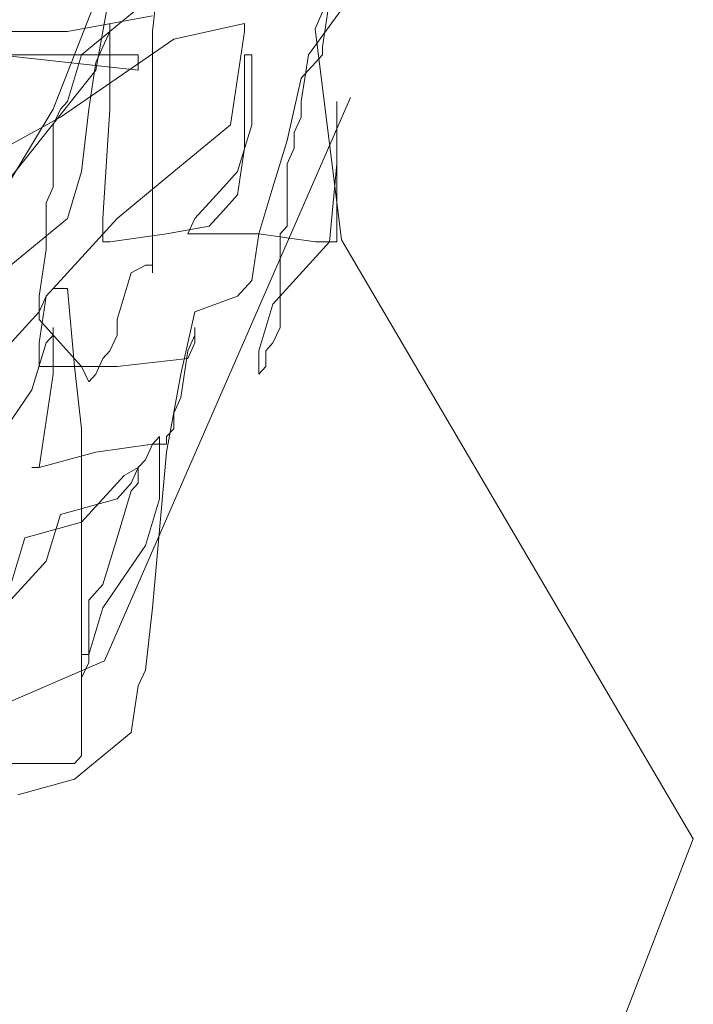
# Model space of a CAD drawing. Units: inches. Extents: x 1994 to 3075, y 3517 to 3950.
# Tile 39 of 58: x 1994.647842 to 1994.650846, y 3553.737497 to 3553.741889. Entities that reach past the tile are written whole.
import ezdxf

# ---------------------------------------------------------------- set-up
doc = ezdxf.new("R2010")
doc.units = ezdxf.units.IN
doc.layers.add('A-FURN-REFR', color=8, linetype='Continuous', lineweight=13)

msp = doc.modelspace()

# ---------------------------------------------------------------- linework, layer by layer
at = {"layer": 'A-FURN-REFR'}
for p, q in [((1994.6505167, 3553.7449295), (1994.6491591, 3553.7418487)), ((1994.6484341, 3553.7418372), (1994.6484657, 3553.7421152)), ((1994.6491295, 3553.741733), (1994.6493823, 3553.7420804)), ((1994.6482444, 3553.742011), (1994.6481812, 3553.7416635)), ((1994.6479915, 3553.7414898), (1994.6481812, 3553.7419762)), ((1994.6491927, 3553.7417677), (1994.6492243, 3553.7419762)), ((1994.6483708, 3553.7419415), (1994.648118, 3553.741733)), ((1994.6480548, 3553.7418372), (1994.6484341, 3553.7419067)), ((1994.6482444, 3553.741872), (1994.6482444, 3553.7414898)), ((1994.6482444, 3553.7418372), (1994.6482444, 3553.741872)), ((1994.648845, 3553.741872), (1994.6485289, 3553.7418025)), ((1994.648845, 3553.7418372), (1994.648845, 3553.741872)), ((1994.6476438, 3553.7418372), (1994.6480548, 3553.7418372)), ((1994.6482128, 3553.7417677), (1994.6482444, 3553.7418372)), ((1994.6484341, 3553.7407601), (1994.6484341, 3553.7418372)), ((1994.6488134, 3553.7416288), (1994.648845, 3553.7418372)), ((1994.6491591, 3553.7418487), (1994.6492772, 3553.7409079)), ((1994.6485289, 3553.7418025), (1994.6480232, 3553.741455)), ((1994.6481812, 3553.7416983), (1994.6482128, 3553.7417677)), ((1994.6491927, 3553.741733), (1994.6491927, 3553.7417677)), ((1994.6477386, 3553.741733), (1994.6483708, 3553.7416635)), ((1994.6483708, 3553.741733), (1994.6478019, 3553.741733)), ((1994.648118, 3553.741733), (1994.6480548, 3553.7415245)), ((1994.6481496, 3553.7414898), (1994.6481812, 3553.7416983)), ((1994.6483708, 3553.7416635), (1994.6483708, 3553.741733)), ((1994.648845, 3553.741733), (1994.6488766, 3553.741733)), ((1994.648845, 3553.741316), (1994.648845, 3553.741733)), ((1994.6488766, 3553.741733), (1994.6488766, 3553.7414202)), ((1994.6490979, 3553.7415245), (1994.6491295, 3553.741733)), ((1994.6490979, 3553.7416288), (1994.6491611, 3553.7416983)), ((1994.6491611, 3553.7416983), (1994.6491927, 3553.741733)), ((1994.6481812, 3553.7416635), (1994.6477386, 3553.7411075)), ((1994.6487818, 3553.7414202), (1994.6488134, 3553.7416288)), ((1994.6490347, 3553.7413508), (1994.6490979, 3553.7416288)), ((1994.6480548, 3553.7415245), (1994.6480232, 3553.7414898)), ((1994.6493179, 3553.7415421), (1994.6482198, 3553.7390294)), ((1994.6490979, 3553.741455), (1994.6490979, 3553.7415245)), ((1994.6492559, 3553.7415245), (1994.6492559, 3553.7412465)), ((1994.6492559, 3553.7408991), (1994.6492559, 3553.7415245)), ((1994.6477386, 3553.7410728), (1994.6479915, 3553.7414898)), ((1994.6480232, 3553.7414898), (1994.6479915, 3553.7414202)), ((1994.648118, 3553.7412118), (1994.6481496, 3553.7414898)), ((1994.6482444, 3553.7414898), (1994.6482128, 3553.7410033)), ((1994.6480232, 3553.741455), (1994.6475174, 3553.741177)), ((1994.6490663, 3553.7413855), (1994.6490979, 3553.741455)), ((1994.6479915, 3553.7414202), (1994.6479915, 3553.7411423)), ((1994.6485289, 3553.7412118), (1994.6487818, 3553.7414202)), ((1994.6488766, 3553.7414202), (1994.6488134, 3553.7412118)), ((1994.6489714, 3553.7411423), (1994.6490347, 3553.7413508)), ((1994.6490663, 3553.741316), (1994.6490663, 3553.7413855)), ((1994.6488134, 3553.7411075), (1994.648845, 3553.741316)), ((1994.6490347, 3553.7412465), (1994.6490663, 3553.741316)), ((1994.6480548, 3553.7410033), (1994.648118, 3553.7412118)), ((1994.648276, 3553.7410033), (1994.6485289, 3553.7412118)), ((1994.6488134, 3553.7412118), (1994.6487501, 3553.7411423)), ((1994.6490347, 3553.7409686), (1994.6490347, 3553.7412465)), ((1994.6492559, 3553.7412465), (1994.6492243, 3553.7408991)), ((1994.6479915, 3553.7411423), (1994.6479599, 3553.7410728)), ((1994.6487501, 3553.7411423), (1994.6486869, 3553.7410728)), ((1994.6489082, 3553.7409338), (1994.6489714, 3553.7411423)), ((1994.6487501, 3553.741038), (1994.6488134, 3553.7411075)), ((1994.6479599, 3553.7410728), (1994.6479599, 3553.7408643)), ((1994.6486869, 3553.7410728), (1994.6486237, 3553.7410033)), ((1994.6486869, 3553.7409686), (1994.6487501, 3553.741038)), ((1994.6478019, 3553.7407948), (1994.6480548, 3553.7410033)), ((1994.6479599, 3553.7406558), (1994.648276, 3553.7410033)), ((1994.6482128, 3553.7410033), (1994.6482128, 3553.7408991)), ((1994.6486237, 3553.7410033), (1994.6485921, 3553.7409338)), ((1994.6484973, 3553.7409338), (1994.6486869, 3553.7409686)), ((1994.649003, 3553.7409338), (1994.6490347, 3553.7409686)), ((1994.6482444, 3553.7408991), (1994.6484973, 3553.7409338)), ((1994.6485921, 3553.7409338), (1994.6489082, 3553.7409338)), ((1994.6488766, 3553.7407253), (1994.6489082, 3553.7409338)), ((1994.6489082, 3553.7409338), (1994.6491611, 3553.7408991)), ((1994.649003, 3553.7405168), (1994.649003, 3553.7409338)), ((1994.6492772, 3553.7409079), (1994.6508462, 3553.7382361)), ((1994.6479599, 3553.7408643), (1994.6479283, 3553.7406558)), ((1994.6482128, 3553.7408991), (1994.6482444, 3553.7408991)), ((1994.6492243, 3553.7408991), (1994.6489714, 3553.7406211)), ((1994.6491611, 3553.7408991), (1994.6492559, 3553.7408991)), ((1994.6483392, 3553.7407601), (1994.6484025, 3553.7407948)), ((1994.6484025, 3553.7407948), (1994.6484341, 3553.7407948)), ((1994.6484341, 3553.7407948), (1994.6484341, 3553.7407601)), ((1994.648276, 3553.7405516), (1994.6483392, 3553.7407601)), ((1994.6479599, 3553.7406558), (1994.6479915, 3553.7406905)), ((1994.6479915, 3553.7406905), (1994.6480548, 3553.7406905)), ((1994.6480548, 3553.7406905), (1994.6480864, 3553.7403431)), ((1994.6488134, 3553.7406558), (1994.6488766, 3553.7407253)), ((1994.6479283, 3553.7405864), (1994.6479599, 3553.7406558)), ((1994.6479283, 3553.7406558), (1994.6479283, 3553.7405516)), ((1994.6479283, 3553.7404473), (1994.6479599, 3553.7406558)), ((1994.6486237, 3553.7405864), (1994.6488134, 3553.7406558)), ((1994.6489714, 3553.7406211), (1994.6489082, 3553.7404126)), ((1994.6477386, 3553.7403778), (1994.6479283, 3553.7405864)), ((1994.6485605, 3553.7403083), (1994.6486237, 3553.7405864)), ((1994.6479283, 3553.7405516), (1994.648118, 3553.7403431)), ((1994.6479915, 3553.7405168), (1994.6479915, 3553.7403083)), ((1994.6479915, 3553.7404821), (1994.6479915, 3553.7405168)), ((1994.648276, 3553.7404821), (1994.648276, 3553.7405516)), ((1994.6486237, 3553.7405168), (1994.6486237, 3553.7404473)), ((1994.6486237, 3553.7404821), (1994.6486237, 3553.7405168)), ((1994.6489714, 3553.7404473), (1994.649003, 3553.7405168)), ((1994.6479599, 3553.7404473), (1994.6479915, 3553.7404821)), ((1994.6482444, 3553.7404126), (1994.648276, 3553.7404821)), ((1994.6485921, 3553.7404126), (1994.6486237, 3553.7404821)), ((1994.6478967, 3553.7402389), (1994.6479599, 3553.7404473)), ((1994.6479283, 3553.7403431), (1994.6479283, 3553.7404473)), ((1994.6486237, 3553.7404473), (1994.6485921, 3553.7403778)), ((1994.6489398, 3553.7404126), (1994.6489714, 3553.7404473)), ((1994.6481812, 3553.7403083), (1994.6482128, 3553.7403778)), ((1994.6482128, 3553.7403778), (1994.6482444, 3553.7404126)), ((1994.6485921, 3553.7403778), (1994.648276, 3553.7403431)), ((1994.6485605, 3553.7402041), (1994.6485921, 3553.7404126)), ((1994.6489082, 3553.7404126), (1994.6489082, 3553.7403083)), ((1994.6489398, 3553.7403431), (1994.6489398, 3553.7404126)), ((1994.648276, 3553.7403431), (1994.6479283, 3553.7403431)), ((1994.6480864, 3553.7403431), (1994.648118, 3553.7400651)), ((1994.648118, 3553.7403431), (1994.6481496, 3553.7402736)), ((1994.6489082, 3553.7403083), (1994.6489398, 3553.7403431)), ((1994.6479915, 3553.7403083), (1994.6479283, 3553.7398914)), ((1994.6481496, 3553.7402736), (1994.6481812, 3553.7403083)), ((1994.6484973, 3553.7399609), (1994.6485605, 3553.7403083)), ((1994.647707, 3553.7399609), (1994.6478967, 3553.7402389)), ((1994.6485289, 3553.7401346), (1994.6485605, 3553.7402041)), ((1994.6485289, 3553.7400651), (1994.6485289, 3553.7401346)), ((1994.648118, 3553.7400651), (1994.648118, 3553.7386057)), ((1994.6484341, 3553.7399956), (1994.6484657, 3553.7400304)), ((1994.6484657, 3553.7400304), (1994.6484657, 3553.7397524)), ((1994.6484973, 3553.7400304), (1994.6485289, 3553.7400651)), ((1994.6484973, 3553.7399956), (1994.6484973, 3553.7400304)), ((1994.6481812, 3553.7399609), (1994.6484341, 3553.7399956)), ((1994.6484025, 3553.7399262), (1994.6484341, 3553.7399956)), ((1994.6484341, 3553.7399956), (1994.6484973, 3553.7399956)), ((1994.6479283, 3553.7398914), (1994.6481812, 3553.7399609)), ((1994.6484341, 3553.7392659), (1994.6484973, 3553.7399609)), ((1994.6483708, 3553.7398914), (1994.6484025, 3553.7399262)), ((1994.6478967, 3553.7398914), (1994.6479283, 3553.7398914)), ((1994.6479283, 3553.7398914), (1994.6478967, 3553.7398914)), ((1994.6483076, 3553.7398567), (1994.648118, 3553.7396481)), ((1994.6483708, 3553.7398914), (1994.6483076, 3553.7398567)), ((1994.6483392, 3553.7398219), (1994.6483708, 3553.7398914)), ((1994.6483708, 3553.7398219), (1994.6483708, 3553.7398914)), ((1994.648276, 3553.7397524), (1994.6483392, 3553.7398219)), ((1994.6483392, 3553.7397872), (1994.6483708, 3553.7398219)), ((1994.648276, 3553.7395786), (1994.6483392, 3553.7397872)), ((1994.6480232, 3553.7396829), (1994.648276, 3553.7397524)), ((1994.6484657, 3553.7397524), (1994.6484025, 3553.7395439)), ((1994.6479599, 3553.7394744), (1994.6480232, 3553.7396829)), ((1994.648118, 3553.7396481), (1994.6478651, 3553.7395786)), ((1994.6478651, 3553.7395786), (1994.6478019, 3553.7393702)), ((1994.6482128, 3553.7393702), (1994.648276, 3553.7395786)), ((1994.6484025, 3553.7395439), (1994.6482128, 3553.7392659)), ((1994.6477703, 3553.7392659), (1994.6479599, 3553.7394744)), ((1994.6481496, 3553.7393007), (1994.6482128, 3553.7393702)), ((1994.6481496, 3553.7390227), (1994.6481496, 3553.7393007)), ((1994.6482128, 3553.7392659), (1994.6481496, 3553.7390575)), ((1994.6484025, 3553.738988), (1994.6484341, 3553.7392659)), ((1994.6482198, 3553.7390294), (1994.6461087, 3553.7381155)), ((1994.648118, 3553.7390575), (1994.648118, 3553.7388837)), ((1994.6481496, 3553.7390575), (1994.648118, 3553.7390575)), ((1994.648118, 3553.7389532), (1994.6481496, 3553.7390227)), ((1994.6483708, 3553.7389184), (1994.6484025, 3553.738988)), ((1994.648118, 3553.7388837), (1994.648118, 3553.7389532)), ((1994.6483392, 3553.73871), (1994.6483708, 3553.7389184)), ((1994.6480864, 3553.7385015), (1994.6483392, 3553.73871)), ((1994.648118, 3553.7386057), (1994.6480864, 3553.738571)), ((1994.6480864, 3553.738571), (1994.6477703, 3553.738571)), ((1994.6478335, 3553.738432), (1994.6480864, 3553.7385015)), ((1994.6508462, 3553.7382361), (1994.6478502, 3553.7304784))]:
    msp.add_line(p, q, dxfattribs=at)

doc.saveas('drawing.dxf')
